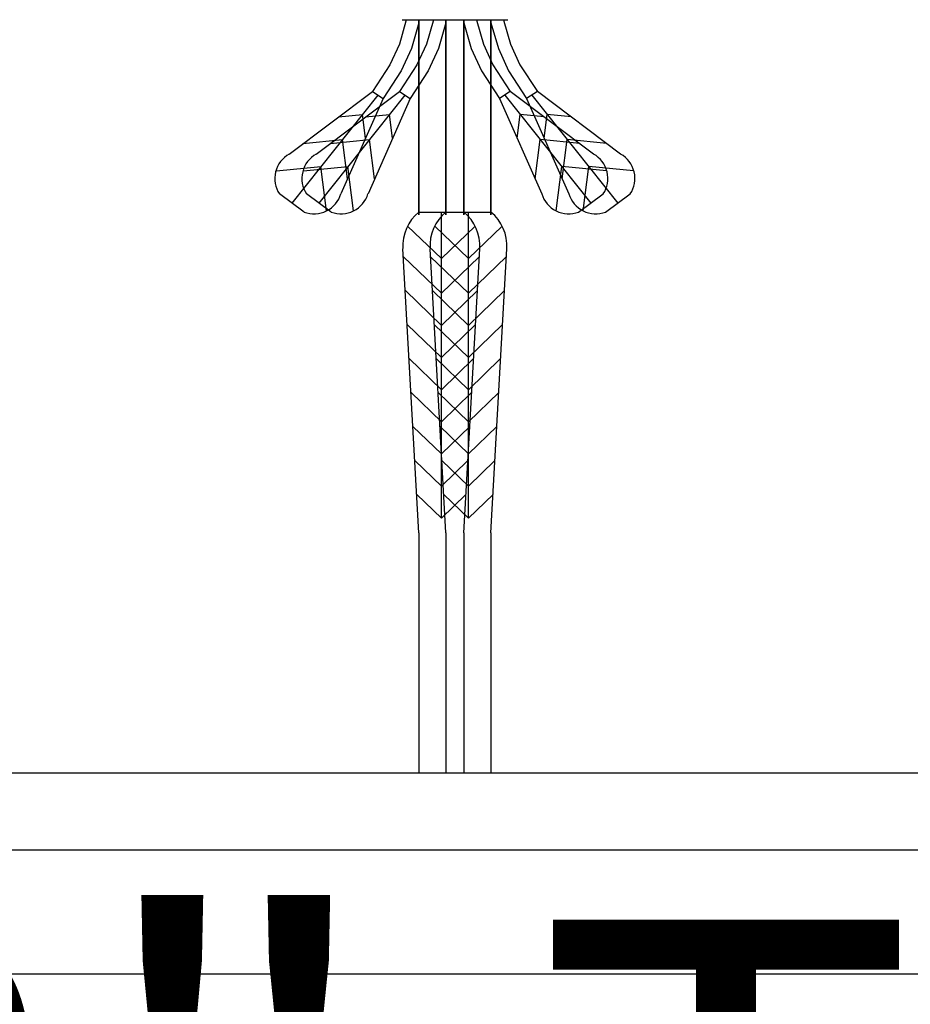
# Model space of a CAD drawing. Units: inches. Extents: x 2278 to 7495, y -71 to 1198.
# Tile 30 of 44: x 5127.04 to 5138.35, y 123.86 to 136.37. Entities that reach past the tile are written whole.
import ezdxf

# ---------------------------------------------------------------- set-up
doc = ezdxf.new("R2010")
doc.units = ezdxf.units.IN
doc.header["$MEASUREMENT"] = 0
doc.layers.add('A-ANNO-DIMS', color=2, linetype='Continuous', lineweight=18)
doc.layers.add('A-ELEV', color=7, linetype='Continuous', lineweight=25)
doc.styles.get("Standard").update_dxf_attribs({"font": 'arial.ttf'})
doc.dimstyles.get("Standard").update_dxf_attribs({"dimtxt": 6, "dimasz": 3, "dimexe": 0.18, "dimexo": 0.0625, "dimgap": 0.09, "dimtad": 0, "dimtih": 1, "dimtoh": 1, "dimdec": 0, "dimzin": 0, "dimdsep": 46, "dimlunit": 3, "dimtxsty": 'Standard', "dimblk": 'ARCHTICK', "dimcen": 0.09, "dimadec": 0, "dimazin": 0, "dimtfac": 1, "dimtdec": 0, "dimtofl": 0, "dimtmove": 0, "dimatfit": 3, "dimfxl": 1, "dimtolj": 1, "dimtzin": 0, "dimarcsym": 0})

# ---------------------------------------------------------------- blocks, each defined once
blk = doc.blocks.new('_ArchTick')
at = {"color": 0, "linetype": 'ByBlock', "const_width": 0.15}
blk.add_lwpolyline([(-0.5, -0.5), (0.5, 0.5)], dxfattribs=at)
blk = doc.blocks.new('*D59')
at = {"layer": 'A-ANNO-DIMS', "color": 0, "lineweight": -2, "transparency": 16777216}
for p, q in [((5096.589, 159.183), (5101.564, 159.183)), ((5101.384, 159.183), (5101.384, 146.185)), ((5101.384, 126.799), (5101.384, 139.796)), ((5096.589, 126.799), (5101.564, 126.799))]:
    blk.add_line(p, q, dxfattribs=at)
at = {"layer": 'Defpoints', "color": 0, "transparency": 16777216}
for p in [(5096.527, 159.183), (5101.384, 159.183), (5096.527, 126.799)]:
    blk.add_point(p, dxfattribs=at)
at = {"layer": 'A-ANNO-DIMS', "color": 0, "lineweight": -2, "transparency": 16777216, "xscale": 3, "yscale": 3, "zscale": 3}
for p, rotation in [((5101.384, 159.183), 90), ((5101.384, 126.799), 270)]:
    blk.add_blockref('_ArchTick', p, dxfattribs=dict(at, rotation=rotation))
at = {"layer": 'A-ANNO-DIMS', "color": 0, "transparency": 16777216, "insert": (5101.384, 142.991), "char_height": 6, "attachment_point": 5}
blk.add_mtext('\\A1;ORNATE BALUSTER 2\'-8 1/2" TYP.', dxfattribs=at)
blk = doc.blocks.new('*D60')
at = {"layer": 'A-ANNO-DIMS', "color": 0, "lineweight": -2, "transparency": 16777216}
for p, q in [((5088.787, 126.736), (5088.787, 121.761)), ((5096.527, 126.736), (5096.527, 121.761)), ((5088.787, 121.941), (5096.527, 121.941)), ((5096.527, 121.941), (5099.527, 121.941))]:
    blk.add_line(p, q, dxfattribs=at)
at = {"layer": 'Defpoints', "color": 0, "transparency": 16777216}
for p in [(5088.787, 126.799), (5096.527, 126.799), (5096.527, 121.941)]:
    blk.add_point(p, dxfattribs=at)
at = {"layer": 'A-ANNO-DIMS', "color": 0, "lineweight": -2, "transparency": 16777216, "xscale": 3, "yscale": 3, "zscale": 3, "rotation": 180}
blk.add_blockref('_ArchTick', (5088.787, 121.941), dxfattribs=at)
at = {"layer": 'A-ANNO-DIMS', "color": 0, "lineweight": -2, "transparency": 16777216, "xscale": 3, "yscale": 3, "zscale": 3}
blk.add_blockref('_ArchTick', (5096.527, 121.941), dxfattribs=at)
at = {"layer": 'A-ANNO-DIMS', "color": 0, "transparency": 16777216, "insert": (5124.894, 121.941), "char_height": 6, "attachment_point": 5}
blk.add_mtext('\\A1;0\'-7 1/2" TYP.', dxfattribs=at)
blk = doc.blocks.new('*D123')
at = {"layer": 'A-ANNO-DIMS', "color": 0, "lineweight": -2, "transparency": 16777216}
for p, q in [((4736.95, 340.157), (4736.95, -23.427)), ((5145.676, -1.81), (5145.676, -23.427)), ((4736.95, -23.247), (4923.929, -23.247)), ((5145.676, -23.247), (4958.697, -23.247))]:
    blk.add_line(p, q, dxfattribs=at)
at = {"layer": 'Defpoints', "color": 0, "transparency": 16777216}
for p in [(4736.95, 340.219), (5145.676, -1.747), (5145.676, -23.247)]:
    blk.add_point(p, dxfattribs=at)
at = {"layer": 'A-ANNO-DIMS', "color": 0, "lineweight": -2, "transparency": 16777216, "xscale": 3, "yscale": 3, "zscale": 3, "rotation": 180}
blk.add_blockref('_ArchTick', (4736.95, -23.247), dxfattribs=at)
at = {"layer": 'A-ANNO-DIMS', "color": 0, "lineweight": -2, "transparency": 16777216, "xscale": 3, "yscale": 3, "zscale": 3}
blk.add_blockref('_ArchTick', (5145.676, -23.247), dxfattribs=at)
at = {"layer": 'A-ANNO-DIMS', "color": 0, "transparency": 16777216, "insert": (4941.313, -23.247), "char_height": 6, "attachment_point": 5}
blk.add_mtext('\\A1;34\'-0 1/2"', dxfattribs=at)
blk = doc.blocks.new('*D131')
at = {"layer": 'A-ANNO-DIMS', "color": 0, "lineweight": -2, "transparency": 16777216}
for p, q in [((5096.176, 99.315), (5096.176, 361.899)), ((5145.676, 118.315), (5145.676, 361.899)), ((5096.176, 361.719), (5105.75, 361.719)), ((5145.676, 361.719), (5136.102, 361.719))]:
    blk.add_line(p, q, dxfattribs=at)
at = {"layer": 'Defpoints', "color": 0, "transparency": 16777216}
for p in [(5145.676, 361.719), (5145.676, 118.253), (5096.176, 99.253)]:
    blk.add_point(p, dxfattribs=at)
at = {"layer": 'A-ANNO-DIMS', "color": 0, "lineweight": -2, "transparency": 16777216, "xscale": 3, "yscale": 3, "zscale": 3, "rotation": 180}
blk.add_blockref('_ArchTick', (5096.176, 361.719), dxfattribs=at)
at = {"layer": 'A-ANNO-DIMS', "color": 0, "lineweight": -2, "transparency": 16777216, "xscale": 3, "yscale": 3, "zscale": 3}
blk.add_blockref('_ArchTick', (5145.676, 361.719), dxfattribs=at)
at = {"layer": 'A-ANNO-DIMS', "color": 0, "transparency": 16777216, "insert": (5120.926, 361.719), "char_height": 6, "attachment_point": 5}
blk.add_mtext('\\A1;4\'-1 1/2"', dxfattribs=at)
blk = doc.blocks.new('*D139')
at = {"layer": 'A-ANNO-DIMS', "color": 0, "lineweight": -2, "transparency": 16777216}
for p, q in [((5092.239, 160.253), (5167.754, 160.253)), ((5167.574, 160.253), (5167.574, 142.408)), ((5167.574, 118.253), (5167.574, 136.097)), ((5145.739, 118.253), (5167.754, 118.253))]:
    blk.add_line(p, q, dxfattribs=at)
at = {"layer": 'Defpoints', "color": 0, "transparency": 16777216}
for p in [(5092.176, 160.253), (5167.574, 160.253), (5145.676, 118.253)]:
    blk.add_point(p, dxfattribs=at)
at = {"layer": 'A-ANNO-DIMS', "color": 0, "lineweight": -2, "transparency": 16777216, "xscale": 3, "yscale": 3, "zscale": 3}
for p, rotation in [((5167.574, 160.253), 90), ((5167.574, 118.253), 270)]:
    blk.add_blockref('_ArchTick', p, dxfattribs=dict(at, rotation=rotation))
at = {"layer": 'A-ANNO-DIMS', "color": 0, "transparency": 16777216, "insert": (5167.574, 139.253), "char_height": 6, "attachment_point": 5}
blk.add_mtext('\\A1;3\'-6"', dxfattribs=at)

msp = doc.modelspace()

# ---------------------------------------------------------------- linework, layer by layer
at = {"layer": 'A-ELEV'}
for p, q in [((5131.947, 136.351), (5131.863, 136.061)), ((5131.897, 136.372), (5132.897, 136.372)), ((5131.947, 136.372), (5131.947, 136.351)), ((5132.111, 136.331), (5132.016, 136.004)), ((5132.11, 136.372), (5132.111, 136.331)), ((5132.111, 136.372), (5132.111, 133.894)), ((5132.111, 133.894), (5132.111, 136.372)), ((5132.291, 136.351), (5132.207, 136.061)), ((5132.24, 136.372), (5133.241, 136.372)), ((5132.29, 136.372), (5132.291, 136.351)), ((5132.455, 136.331), (5132.36, 136.004)), ((5132.454, 136.372), (5132.455, 136.331)), ((5132.455, 136.372), (5132.455, 133.894)), ((5132.455, 133.894), (5132.455, 136.372)), ((5132.682, 136.372), (5132.682, 133.894)), ((5132.682, 133.894), (5132.682, 136.372)), ((5132.684, 136.372), (5132.682, 136.331)), ((5132.682, 136.331), (5132.777, 136.004)), ((5132.847, 136.372), (5132.846, 136.351)), ((5132.846, 136.351), (5132.93, 136.061)), ((5133.026, 136.372), (5133.026, 133.894)), ((5133.026, 133.894), (5133.026, 136.372)), ((5133.027, 136.372), (5133.026, 136.331)), ((5133.026, 136.331), (5133.121, 136.004)), ((5133.191, 136.372), (5133.19, 136.351)), ((5133.19, 136.351), (5133.274, 136.061)), ((5131.863, 136.061), (5131.743, 135.8)), ((5132.016, 136.004), (5131.886, 135.721)), ((5132.207, 136.061), (5132.087, 135.8)), ((5132.36, 136.004), (5132.23, 135.721)), ((5132.777, 136.004), (5132.907, 135.721)), ((5132.93, 136.061), (5133.05, 135.8)), ((5133.121, 136.004), (5133.251, 135.721)), ((5133.274, 136.061), (5133.394, 135.8)), ((5131.743, 135.8), (5131.521, 135.459)), ((5131.886, 135.721), (5131.658, 135.37)), ((5132.087, 135.8), (5131.865, 135.459)), ((5132.23, 135.721), (5132.002, 135.37)), ((5132.907, 135.721), (5133.135, 135.37)), ((5133.05, 135.8), (5133.272, 135.459)), ((5133.251, 135.721), (5133.479, 135.37)), ((5133.394, 135.8), (5133.616, 135.459)), ((5130.463, 134.665), (5131.521, 135.459)), ((5130.807, 134.665), (5131.865, 135.459)), ((5131.521, 135.459), (5131.658, 135.37)), ((5131.865, 135.459), (5132.002, 135.37)), ((5133.272, 135.459), (5133.135, 135.37)), ((5134.33, 134.665), (5133.272, 135.459)), ((5133.616, 135.459), (5133.479, 135.37)), ((5134.674, 134.665), (5133.616, 135.459)), ((5131.59, 135.414), (5130.497, 134.043)), ((5131.934, 135.414), (5130.841, 134.043)), ((5131.658, 135.37), (5131.121, 134.161)), ((5132.002, 135.37), (5131.465, 134.161)), ((5133.135, 135.37), (5133.672, 134.161)), ((5133.203, 135.414), (5134.296, 134.043)), ((5133.479, 135.37), (5134.016, 134.161)), ((5133.547, 135.414), (5134.64, 134.043)), ((5131.089, 135.139), (5131.394, 135.169)), ((5131.434, 134.865), (5131.394, 135.169)), ((5131.433, 135.139), (5131.738, 135.169)), ((5131.778, 134.865), (5131.738, 135.169)), ((5133.359, 134.865), (5133.399, 135.169)), ((5133.704, 135.139), (5133.399, 135.169)), ((5133.703, 134.865), (5133.743, 135.169)), ((5134.048, 135.139), (5133.743, 135.169)), ((5130.638, 134.801), (5131.14, 134.85)), ((5130.982, 134.801), (5131.484, 134.85)), ((5131.205, 134.35), (5131.14, 134.85)), ((5131.549, 134.35), (5131.484, 134.85)), ((5133.588, 134.35), (5133.653, 134.85)), ((5134.155, 134.801), (5133.653, 134.85)), ((5133.932, 134.35), (5133.997, 134.85)), ((5134.499, 134.801), (5133.997, 134.85)), ((5130.301, 134.45), (5130.865, 134.505)), ((5130.645, 134.45), (5131.209, 134.505)), ((5130.938, 133.942), (5130.865, 134.505)), ((5131.282, 133.942), (5131.209, 134.505)), ((5133.855, 133.942), (5133.928, 134.505)), ((5134.493, 134.45), (5133.928, 134.505)), ((5134.199, 133.942), (5134.272, 134.505)), ((5134.836, 134.45), (5134.272, 134.505)), ((5130.654, 133.927), (5130.34, 134.158)), ((5130.998, 133.927), (5130.684, 134.158)), ((5134.139, 133.927), (5134.453, 134.158)), ((5134.483, 133.927), (5134.797, 134.158)), ((5132.111, 133.927), (5132.682, 133.927)), ((5132.397, 130.039), (5132.397, 133.927)), ((5132.455, 133.927), (5133.026, 133.927)), ((5132.74, 130.039), (5132.74, 133.927)), ((5131.968, 133.751), (5132.397, 133.337)), ((5132.312, 133.751), (5132.74, 133.337)), ((5132.825, 133.751), (5132.397, 133.337)), ((5133.169, 133.751), (5132.74, 133.337)), ((5132.111, 129.854), (5131.909, 133.463)), ((5132.455, 129.854), (5132.253, 133.463)), ((5132.682, 129.854), (5132.884, 133.463)), ((5133.026, 129.854), (5133.228, 133.463)), ((5131.915, 133.361), (5132.397, 132.896)), ((5132.259, 133.361), (5132.74, 132.896)), ((5132.878, 133.361), (5132.397, 132.896)), ((5133.222, 133.361), (5132.74, 132.896)), ((5131.939, 132.93), (5132.397, 132.488)), ((5132.283, 132.93), (5132.74, 132.488)), ((5132.854, 132.93), (5132.397, 132.488)), ((5133.198, 132.93), (5132.74, 132.488)), ((5131.963, 132.498), (5132.397, 132.079)), ((5132.307, 132.498), (5132.74, 132.079)), ((5132.83, 132.498), (5132.397, 132.079)), ((5133.174, 132.498), (5132.74, 132.079)), ((5131.987, 132.067), (5132.397, 131.671)), ((5132.331, 132.067), (5132.74, 131.671)), ((5132.806, 132.067), (5132.397, 131.671)), ((5133.15, 132.067), (5132.74, 131.671)), ((5132.012, 131.635), (5132.397, 131.263)), ((5132.356, 131.635), (5132.74, 131.263)), ((5132.781, 131.635), (5132.397, 131.263)), ((5133.125, 131.635), (5132.74, 131.263)), ((5132.036, 131.204), (5132.397, 130.855)), ((5132.38, 131.204), (5132.74, 130.855)), ((5132.757, 131.204), (5132.397, 130.855)), ((5133.101, 131.204), (5132.74, 130.855)), ((5132.06, 130.772), (5132.397, 130.447)), ((5132.733, 130.772), (5132.397, 130.447)), ((5132.404, 130.772), (5132.74, 130.447)), ((5133.077, 130.772), (5132.74, 130.447)), ((5132.084, 130.341), (5132.397, 130.039)), ((5132.709, 130.341), (5132.397, 130.039)), ((5132.428, 130.341), (5132.74, 130.039)), ((5133.053, 130.341), (5132.74, 130.039)), ((5132.111, 129.854), (5132.111, 126.799)), ((5132.455, 129.854), (5132.455, 126.799)), ((5132.682, 129.854), (5132.682, 126.799)), ((5133.026, 129.854), (5133.026, 126.799)), ((5145.676, 126.799), (5066.016, 126.799)), ((5145.676, 125.821), (5066.016, 125.821)), ((4874.676, 124.253), (5145.676, 124.253))]:
    msp.add_line(p, q, dxfattribs=at)
for centre, radius, start, end in [((5130.637, 134.354), 0.356, 119.3212, 213.425), ((5130.981, 134.354), 0.356, 119.3212, 213.425), ((5134.156, 134.354), 0.356, 326.575, 60.6788), ((5134.5, 134.354), 0.356, 326.575, 60.6788), ((5130.779, 134.261), 0.356, 249.4937, 343.5975), ((5131.123, 134.261), 0.356, 249.4937, 343.5975), ((5134.014, 134.261), 0.356, 196.4025, 290.5063), ((5134.358, 134.261), 0.356, 196.4025, 290.5063), ((5132.455, 133.502), 0.547, 128.9283, 183.9822), ((5132.799, 133.502), 0.547, 128.9283, 183.9822), ((5132.338, 133.502), 0.547, 356.0178, 51.0717), ((5132.682, 133.502), 0.547, 356.0178, 51.0717)]:
    msp.add_arc(centre, radius, start, end, dxfattribs=at)

# ---------------------------------------------------------------- dimensions: what is measured, and where the dimension line sits
at = {"layer": 'A-ANNO-DIMS'}
for base, p1, p2, picture, middle in [((5145.676, 361.719), (5096.176, 99.253), (5145.676, 118.253), '*D131', (5120.926, 361.719)), ((5145.676, -23.247), (4736.95, 340.219), (5145.676, -1.747), '*D123', (4941.313, -23.247))]:
    dim = msp.add_linear_dim(base=base, p1=p1, p2=p2, dimstyle='Standard', override={"dimdec": 1, "dimlfac": 1, "dimrnd": 0, "dimzin": 1, "dimdsep": 46, "dimlunit": 4, "dimfrac": 2}, dxfattribs=at)
    dim.commit()
    dim.dimension.update_dxf_attribs({"geometry": picture, "text_midpoint": middle})
dim = msp.add_linear_dim(base=(5101.384, 159.183), p1=(5096.527, 126.799), p2=(5096.527, 159.183), angle=90, text='ORNATE BALUSTER <> TYP.', dimstyle='Standard', override={"dimdec": 1, "dimrnd": 0, "dimzin": 1, "dimlunit": 4, "dimfrac": 2}, dxfattribs=at)
dim.commit()
dim.dimension.update_dxf_attribs({"geometry": '*D59', "text_midpoint": (5101.384, 142.991)})
dim = msp.add_linear_dim(base=(5167.574, 160.253), p1=(5145.676, 118.253), p2=(5092.176, 160.253), angle=90, dimstyle='Standard', override={"dimdec": 1, "dimlfac": 1, "dimrnd": 0, "dimzin": 1, "dimdsep": 46, "dimlunit": 4, "dimfrac": 2}, dxfattribs=at)
dim.commit()
dim.dimension.update_dxf_attribs({"geometry": '*D139', "text_midpoint": (5167.574, 139.253)})
dim = msp.add_linear_dim(base=(5096.527, 121.941), p1=(5088.787, 126.799), p2=(5096.527, 126.799), text='<> TYP.', dimstyle='Standard', override={"dimdec": 1, "dimrnd": 0, "dimzin": 1, "dimlunit": 4, "dimfrac": 2}, dxfattribs=at)
dim.commit()
dim.dimension.update_dxf_attribs({"geometry": '*D60', "text_midpoint": (5124.894, 121.941)})

doc.saveas('drawing.dxf')
